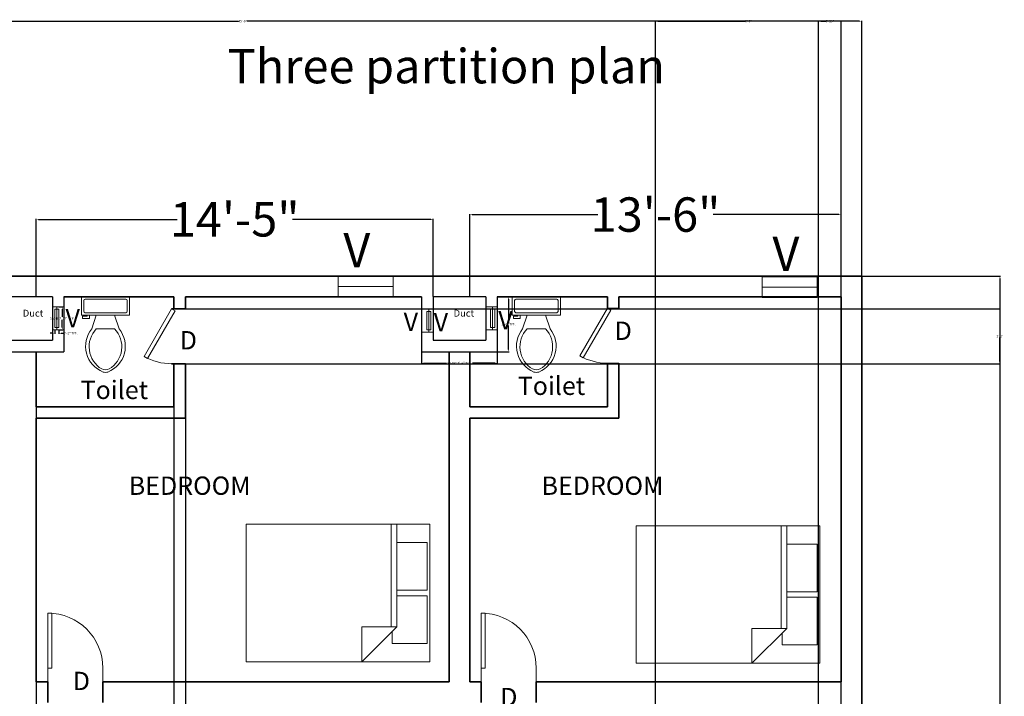
# Model space of a CAD drawing. Units: inches. Extents: x 371 to 1095, y -45 to 1219.
# Tile 18 of 18: x 666 to 1095, y 799 to 1094. Entities that reach past the tile are written whole.
import ezdxf

# ---------------------------------------------------------------- set-up
doc = ezdxf.new("R2010")
doc.units = ezdxf.units.IN
doc.header["$MEASUREMENT"] = 0
for name, color, linetype, lineweight in [('A-ANNO-DIMS', 2, 'Continuous', 18), ('A-ANNO-TEXT', 7, 'Continuous', 18), ('A-AREA-IDEN', 7, 'Continuous', 18), ('A-DOOR', 3, 'Continuous', 18), ('A-FLOR-FIXT', 9, 'Continuous', 18), ('A-FLOR-SHFT', 7, 'Continuous', 25), ('A-FURN', 254, 'Continuous', 18), ('A-GLAZ', 4, 'Continuous', 18), ('A-WALL', 40, 'Continuous', 35)]:
    doc.layers.add(name, color=color, linetype=linetype, lineweight=lineweight)
doc.styles.get("Standard").update_dxf_attribs({"font": 'arial.ttf'})
doc.dimstyles.get("Standard").update_dxf_attribs({"dimtxt": 1, "dimasz": 1, "dimexe": 0.18, "dimexo": 0.0625, "dimgap": 0.09, "dimtad": 0, "dimtih": 1, "dimtoh": 1, "dimdec": 0, "dimzin": 0, "dimdsep": 46, "dimlunit": 3, "dimtxsty": 'Standard', "dimcen": 0.09, "dimadec": 0, "dimazin": 0, "dimtfac": 1, "dimtdec": 0, "dimtofl": 0, "dimtmove": 0, "dimatfit": 3, "dimfxl": 1, "dimtolj": 1, "dimtzin": 0, "dimarcsym": 0})

# ---------------------------------------------------------------- blocks, each defined once
blk = doc.blocks.new('*U2')
for p, q in [((9.5, -6), (9.5, -2)), ((-10, -8.5), (-8, -8.5)), ((-10, -9.5), (-10, -8.5)), ((-8, -8.5), (-8, -8)), ((-7, -8), (-7, -9.5)), ((-4, -8), (-6, -14)), ((4, -8), (6, -14)), ((-7, -9.5), (-10, -9.5)), ((4, -14), (-4, -14))]:
    blk.add_line(p, q)
blk.add_lwpolyline([(10.5, -8), (10.5, 0), (-10.5, 0), (-10.5, -8)], close=True)
for points in [[(-9.5, -2), (-9.5, -6)], [(8.5, -1), (-8.5, -1)], [(-8.5, -7), (8.5, -7)]]:
    blk.add_lwpolyline(points)
for centre, radius, start, end in [((-8.62, -1.88), 0.884, 81.8699, 188.1301), ((8.62, -1.88), 0.884, 351.8699, 98.1301), ((-8.62, -6.12), 0.884, 171.8699, 278.1301), ((8.62, -6.12), 0.884, 261.8699, 8.1301), ((3.52, -21.58), 12.17, 141.4691, 247.9714), ((4.2, -21.82), 11.33, 136.3677, 238.9468), ((-3.52, -21.58), 12.17, 292.0284, 38.5307), ((-4.2, -21.82), 11.33, 301.053, 43.6321), ((0, -27.88), 4, 245.7318, 294.2682), ((0, -29), 4, 254.8605, 285.1395)]:
    blk.add_arc(centre, radius, start, end)
blk = doc.blocks.new('*U6')
for p, q in [((0, 0), (0, 6)), ((24, 0), (24, 6))]:
    blk.add_line(p, q)
blk.add_lwpolyline([(0, 0), (20.78, -12), (21.66, -10.48), (0.87, 1.52)], close=True)
blk.add_arc((0, 0), 24, 330, 0)
blk = doc.blocks.new('*U7')
for p, q in [((0, 0), (0, 5)), ((24, 0), (24, 5))]:
    blk.add_line(p, q)
blk.add_lwpolyline([(0, 0), (20.78, -12), (21.66, -10.48), (0.87, 1.52)], close=True)
blk.add_arc((0, 0), 24, 330, 0)
blk = doc.blocks.new('*U4')
for p, q in [((-24, 0), (-24, -6)), ((0, 0), (0, -6))]:
    blk.add_line(p, q)
blk.add_lwpolyline([(0, 0), (0, 24), (-1.75, 24), (-1.75, 0)], close=True)
blk.add_arc((0, 0), 24, 90, 180)
blk = doc.blocks.new('*D9')
at = {"layer": 'A-ANNO-DIMS', "color": 0, "lineweight": -2, "transparency": 16777216}
for p, q in [((672.81, 973.09), (672.81, 1006.96)), ((673.81, 1006.78), (734.16, 1006.78)), ((844.81, 1006.78), (784.46, 1006.78)), ((845.81, 973.09), (845.81, 1006.96))]:
    blk.add_line(p, q, dxfattribs=at)
at = {"layer": 'A-ANNO-DIMS', "color": 0, "transparency": 16777216}
for points in [[(673.81, 1006.95), (673.81, 1006.61), (672.81, 1006.78)], [(844.81, 1006.95), (844.81, 1006.61), (845.81, 1006.78)]]:
    blk.add_solid(points, dxfattribs=at)
at = {"layer": 'Defpoints', "color": 0, "transparency": 16777216}
for p in [(845.81, 1006.78), (672.81, 973.03), (845.81, 973.03)]:
    blk.add_point(p, dxfattribs=at)
at = {"layer": 'A-ANNO-DIMS', "color": 0, "transparency": 16777216, "insert": (759.31, 1006.78), "char_height": 1, "attachment_point": 5}
blk.add_mtext('\\A1;{\\H15x;14\'-5"}', dxfattribs=at)
blk = doc.blocks.new('*D10')
at = {"layer": 'A-ANNO-DIMS', "color": 0, "lineweight": -2, "transparency": 16777216}
for p, q in [((861.81, 973.2), (861.81, 1009.05)), ((1023.81, 973.09), (1023.81, 1009.05)), ((862.81, 1008.87), (917.66, 1008.87)), ((1022.81, 1008.87), (967.96, 1008.87))]:
    blk.add_line(p, q, dxfattribs=at)
at = {"layer": 'A-ANNO-DIMS', "color": 0, "transparency": 16777216}
for points in [[(862.81, 1009.03), (862.81, 1008.7), (861.81, 1008.87)], [(1022.81, 1009.03), (1022.81, 1008.7), (1023.81, 1008.87)]]:
    blk.add_solid(points, dxfattribs=at)
at = {"layer": 'Defpoints', "color": 0, "transparency": 16777216}
for p in [(1023.81, 1008.87), (861.81, 973.14), (1023.81, 973.03)]:
    blk.add_point(p, dxfattribs=at)
at = {"layer": 'A-ANNO-DIMS', "color": 0, "transparency": 16777216, "insert": (942.81, 1008.87), "char_height": 1, "attachment_point": 5}
blk.add_mtext('\\A1;{\\H15x;13\'-6"}', dxfattribs=at)
blk = doc.blocks.new('Bed - Queen')
for p, q in [((0, -80.00003), (0, 0)), ((0, 0), (59.99999, 0)), ((59.99999, 0), (59.99999, -80.00003)), ((7.99999, -1.2), (28.79998, -1.2)), ((7.99999, -14.4), (7.99999, -1.2)), ((28.79998, -1.2), (28.79998, -14.4)), ((31.19999, -1.2), (51.99999, -1.2)), ((31.19999, -14.4), (31.19999, -1.2)), ((51.99999, -1.2), (51.99999, -16.4)), ((0, -14.4), (44.8, -14.4)), ((44.8, -16.8), (0, -16.8)), ((59.99999, -29.6), (44.8, -14.4)), ((44.8, -14.4), (44.8, -29.6)), ((51.99999, -16.4), (46.79936, -16.4)), ((44.8, -29.6), (59.99999, -29.6)), ((59.99999, -80.00003), (0, -80.00003))]:
    blk.add_line(p, q)
blk = doc.blocks.new('VENT-24-REAR')
blk.add_line((0, 4.5), (24, 4.5))
blk.add_lwpolyline([(0, 9), (24, 9), (24, 0), (0, 0)], close=True)
blk = doc.blocks.new('VENT-DUCT-SASH')
blk.add_line((0.9, 10), (0.9, 0))
blk.add_lwpolyline([(1.79, 9), (1.79, 1), (0, 1), (0, 9)], close=True)
blk = doc.blocks.new('SHAFT-REAR')
for p, q in [((0, 24), (0, 0)), ((5, 24), (5, 5)), ((28, 24), (5, 24)), ((28, 24), (28, 5)), ((33, 24), (33, 0)), ((5, 5), (28, 5)), ((0, 0), (33, 0))]:
    blk.add_line(p, q)
blk = doc.blocks.new('*D42')
at = {"layer": 'A-ANNO-DIMS', "color": 0, "lineweight": -2, "transparency": 16777216}
for p, q in [((682.69, 968.59), (684.31, 968.59)), ((684.13, 967.59), (684.13, 964.19)), ((684.13, 959.59), (684.13, 962.98)), ((682.69, 958.59), (684.31, 958.59))]:
    blk.add_line(p, q, dxfattribs=at)
at = {"layer": 'A-ANNO-DIMS', "color": 0, "transparency": 16777216}
for points in [[(683.96, 967.59), (684.3, 967.59), (684.13, 968.59)], [(683.96, 959.59), (684.3, 959.59), (684.13, 958.59)]]:
    blk.add_solid(points, dxfattribs=at)
at = {"layer": 'Defpoints', "color": 0, "transparency": 16777216}
for p in [(682.63, 968.59), (684.13, 968.59), (682.63, 958.59)]:
    blk.add_point(p, dxfattribs=at)
at = {"layer": 'A-ANNO-DIMS', "color": 0, "transparency": 16777216, "insert": (684.13, 963.59), "char_height": 1, "attachment_point": 5}
blk.add_mtext('\\A1;SASH 0\'-10" TYP.', dxfattribs=at)
blk = doc.blocks.new('*D43')
at = {"layer": 'A-ANNO-DIMS', "color": 0, "lineweight": -2, "transparency": 16777216}
for p, q in [((680.84, 958.52), (680.84, 956.91)), ((682.63, 958.52), (682.63, 956.91)), ((679.84, 957.09), (678.84, 957.09)), ((683.63, 957.09), (684.63, 957.09))]:
    blk.add_line(p, q, dxfattribs=at)
at = {"layer": 'A-ANNO-DIMS', "color": 0, "transparency": 16777216}
for points in [[(679.84, 957.25), (679.84, 956.92), (680.84, 957.09)], [(683.63, 957.25), (683.63, 956.92), (682.63, 957.09)]]:
    blk.add_solid(points, dxfattribs=at)
at = {"layer": 'Defpoints', "color": 0, "transparency": 16777216}
for p in [(680.84, 958.59), (682.63, 958.59), (682.63, 957.09)]:
    blk.add_point(p, dxfattribs=at)
at = {"layer": 'A-ANNO-DIMS', "color": 0, "transparency": 16777216, "insert": (687.77, 957.09), "char_height": 1, "attachment_point": 5}
blk.add_mtext('\\A1;0\'-2" TYP.', dxfattribs=at)
blk = doc.blocks.new('*D46')
at = {"layer": 'A-ANNO-DIMS', "color": 0, "lineweight": -2, "transparency": 16777216}
for p, q in [((840.81, 948.96), (840.81, 943.9)), ((873.81, 948.96), (873.81, 943.9)), ((841.81, 944.08), (851.69, 944.08)), ((872.81, 944.08), (862.93, 944.08))]:
    blk.add_line(p, q, dxfattribs=at)
at = {"layer": 'A-ANNO-DIMS', "color": 0, "transparency": 16777216}
for points in [[(841.81, 944.24), (841.81, 943.91), (840.81, 944.08)], [(872.81, 944.24), (872.81, 943.91), (873.81, 944.08)]]:
    blk.add_solid(points, dxfattribs=at)
at = {"layer": 'Defpoints', "color": 0, "transparency": 16777216}
for p in [(840.81, 949.03), (873.81, 949.03), (873.81, 944.08)]:
    blk.add_point(p, dxfattribs=at)
at = {"layer": 'A-ANNO-DIMS', "color": 0, "transparency": 16777216, "insert": (857.31, 944.08), "char_height": 1, "attachment_point": 5}
blk.add_mtext('\\A1;SHAFT 2\'-9" TYP.', dxfattribs=at)
blk = doc.blocks.new('*D47')
at = {"layer": 'A-ANNO-DIMS', "color": 0, "lineweight": -2, "transparency": 16777216}
for p, q in [((873.87, 973.03), (878.94, 973.03)), ((878.76, 972.03), (878.76, 961.63)), ((878.76, 950.03), (878.76, 960.42)), ((873.87, 949.03), (878.94, 949.03))]:
    blk.add_line(p, q, dxfattribs=at)
at = {"layer": 'A-ANNO-DIMS', "color": 0, "transparency": 16777216}
for points in [[(878.59, 972.03), (878.92, 972.03), (878.76, 973.03)], [(878.59, 950.03), (878.92, 950.03), (878.76, 949.03)]]:
    blk.add_solid(points, dxfattribs=at)
at = {"layer": 'Defpoints', "color": 0, "transparency": 16777216}
for p in [(873.81, 973.03), (878.76, 973.03), (873.81, 949.03)]:
    blk.add_point(p, dxfattribs=at)
at = {"layer": 'A-ANNO-DIMS', "color": 0, "transparency": 16777216, "insert": (878.76, 961.03), "char_height": 1, "attachment_point": 5}
blk.add_mtext('\\A1;2\'-0" TYP.', dxfattribs=at)
blk = doc.blocks.new('*D50')
at = {"layer": 'A-ANNO-DIMS', "color": 0, "lineweight": -2, "transparency": 16777216}
for p, q in [((492.81, 982.09), (492.81, 1093.41)), ((493.81, 1093.23), (760.98, 1093.23)), ((1031.81, 1093.23), (764.64, 1093.23)), ((1032.81, 982.09), (1032.81, 1093.41))]:
    blk.add_line(p, q, dxfattribs=at)
at = {"layer": 'A-ANNO-DIMS', "color": 0, "transparency": 16777216}
for points in [[(493.81, 1093.39), (493.81, 1093.06), (492.81, 1093.23)], [(1031.81, 1093.39), (1031.81, 1093.06), (1032.81, 1093.23)]]:
    blk.add_solid(points, dxfattribs=at)
at = {"layer": 'Defpoints', "color": 0, "transparency": 16777216}
for p in [(1032.81, 1093.23), (492.81, 982.03), (1032.81, 982.03)]:
    blk.add_point(p, dxfattribs=at)
at = {"layer": 'A-ANNO-DIMS', "color": 0, "transparency": 16777216, "insert": (762.81, 1093.23), "char_height": 1, "attachment_point": 5}
blk.add_mtext('\\A1;45\'-0"', dxfattribs=at)
blk = doc.blocks.new('*D51')
at = {"layer": 'A-ANNO-DIMS', "color": 0, "lineweight": -2, "transparency": 16777216}
for p, q in [((1032.87, 982.03), (1093.19, 982.03)), ((1093.01, 981.03), (1093.01, 532.63)), ((1093.01, 83.03), (1093.01, 531.42)), ((1032.87, 82.03), (1093.19, 82.03))]:
    blk.add_line(p, q, dxfattribs=at)
at = {"layer": 'A-ANNO-DIMS', "color": 0, "transparency": 16777216}
for points in [[(1092.84, 981.03), (1093.17, 981.03), (1093.01, 982.03)], [(1092.84, 83.03), (1093.17, 83.03), (1093.01, 82.03)]]:
    blk.add_solid(points, dxfattribs=at)
at = {"layer": 'Defpoints', "color": 0, "transparency": 16777216}
for p in [(1032.81, 982.03), (1093.01, 982.03), (1032.81, 82.03)]:
    blk.add_point(p, dxfattribs=at)
at = {"layer": 'A-ANNO-DIMS', "color": 0, "transparency": 16777216, "insert": (1093.01, 532.03), "char_height": 1, "attachment_point": 5}
blk.add_mtext('\\A1;75\'-0"', dxfattribs=at)
blk = doc.blocks.new('*D54')
at = {"layer": 'A-ANNO-DIMS', "color": 0, "lineweight": -2, "transparency": 16777216}
for p, q in [((672.81, 924.96), (672.81, -43.83)), ((732.81, 924.96), (732.81, -43.83)), ((673.81, -43.65), (701.39, -43.65)), ((731.81, -43.65), (704.23, -43.65))]:
    blk.add_line(p, q, dxfattribs=at)
at = {"layer": 'A-ANNO-DIMS', "color": 0, "transparency": 16777216}
for points in [[(673.81, -43.48), (673.81, -43.82), (672.81, -43.65)], [(731.81, -43.48), (731.81, -43.82), (732.81, -43.65)]]:
    blk.add_solid(points, dxfattribs=at)
at = {"layer": 'Defpoints', "color": 0, "transparency": 16777216}
for p in [(672.81, 925.03), (732.81, 925.03), (732.81, -43.65)]:
    blk.add_point(p, dxfattribs=at)
at = {"layer": 'A-ANNO-DIMS', "color": 0, "transparency": 16777216, "insert": (702.81, -43.65), "char_height": 1, "attachment_point": 5}
blk.add_mtext('\\A1;5\'-0"', dxfattribs=at)
blk = doc.blocks.new('*D56')
at = {"layer": 'A-ANNO-DIMS', "color": 0, "lineweight": -2, "transparency": 16777216}
for p, q in [((737.87, 967.8), (1093.19, 967.8)), ((1093.01, 966.8), (1093.01, 956.4)), ((1093.01, 944.8), (1093.01, 955.2)), ((737.87, 943.8), (1093.19, 943.8))]:
    blk.add_line(p, q, dxfattribs=at)
at = {"layer": 'A-ANNO-DIMS', "color": 0, "transparency": 16777216}
for points in [[(1092.84, 966.8), (1093.17, 966.8), (1093.01, 967.8)], [(1092.84, 944.8), (1093.17, 944.8), (1093.01, 943.8)]]:
    blk.add_solid(points, dxfattribs=at)
at = {"layer": 'Defpoints', "color": 0, "transparency": 16777216}
for p in [(737.81, 967.8), (1093.01, 967.8), (737.81, 943.8)]:
    blk.add_point(p, dxfattribs=at)
at = {"layer": 'A-ANNO-DIMS', "color": 0, "transparency": 16777216, "insert": (1093.01, 955.8), "char_height": 1, "attachment_point": 5}
blk.add_mtext('\\A1;2\'-0"', dxfattribs=at)
blk = doc.blocks.new('*D57')
at = {"layer": 'A-ANNO-DIMS', "color": 0, "lineweight": -2, "transparency": 16777216}
for p, q in [((732.81, 924.96), (732.81, -43.83)), ((737.81, 919.96), (737.81, -43.83)), ((731.81, -43.65), (730.81, -43.65)), ((738.81, -43.65), (739.81, -43.65))]:
    blk.add_line(p, q, dxfattribs=at)
at = {"layer": 'A-ANNO-DIMS', "color": 0, "transparency": 16777216}
for points in [[(731.81, -43.48), (731.81, -43.82), (732.81, -43.65)], [(738.81, -43.48), (738.81, -43.82), (737.81, -43.65)]]:
    blk.add_solid(points, dxfattribs=at)
at = {"layer": 'Defpoints', "color": 0, "transparency": 16777216}
for p in [(732.81, 925.03), (737.81, 920.03), (732.81, -43.65)]:
    blk.add_point(p, dxfattribs=at)
at = {"layer": 'A-ANNO-DIMS', "color": 0, "transparency": 16777216, "insert": (735.31, -43.65), "char_height": 1, "attachment_point": 5}
blk.add_mtext('\\A1;0\'-5"', dxfattribs=at)
blk = doc.blocks.new('*D63')
at = {"layer": 'A-ANNO-DIMS', "color": 0, "lineweight": -2, "transparency": 16777216}
for p, q in [((942.81, 580.09), (942.81, 1093.41)), ((943.81, 1093.23), (981.89, 1093.23)), ((1022.81, 1093.23), (984.73, 1093.23)), ((1023.81, 580.09), (1023.81, 1093.41))]:
    blk.add_line(p, q, dxfattribs=at)
at = {"layer": 'A-ANNO-DIMS', "color": 0, "transparency": 16777216}
for points in [[(943.81, 1093.39), (943.81, 1093.06), (942.81, 1093.23)], [(1022.81, 1093.39), (1022.81, 1093.06), (1023.81, 1093.23)]]:
    blk.add_solid(points, dxfattribs=at)
at = {"layer": 'Defpoints', "color": 0, "transparency": 16777216}
for p in [(1023.81, 1093.23), (942.81, 580.03), (1023.81, 580.03)]:
    blk.add_point(p, dxfattribs=at)
at = {"layer": 'A-ANNO-DIMS', "color": 0, "transparency": 16777216, "insert": (983.31, 1093.23), "char_height": 1, "attachment_point": 5}
blk.add_mtext('\\A1;6\'-9"', dxfattribs=at)
blk = doc.blocks.new('*D64')
at = {"layer": 'A-ANNO-DIMS', "color": 0, "lineweight": -2, "transparency": 16777216}
for p, q in [((1013.84, 464.01), (1013.84, 1093.41)), ((1014.84, 1093.23), (1017.01, 1093.23)), ((1022.81, 1093.23), (1020.63, 1093.23)), ((1023.81, 451.09), (1023.81, 1093.41))]:
    blk.add_line(p, q, dxfattribs=at)
at = {"layer": 'A-ANNO-DIMS', "color": 0, "transparency": 16777216}
for points in [[(1014.84, 1093.39), (1014.84, 1093.06), (1013.84, 1093.23)], [(1022.81, 1093.39), (1022.81, 1093.06), (1023.81, 1093.23)]]:
    blk.add_solid(points, dxfattribs=at)
at = {"layer": 'Defpoints', "color": 0, "transparency": 16777216}
for p in [(1023.81, 1093.23), (1013.84, 463.94), (1023.81, 451.03)]:
    blk.add_point(p, dxfattribs=at)
at = {"layer": 'A-ANNO-DIMS', "color": 0, "transparency": 16777216, "insert": (1018.82, 1093.23), "char_height": 1, "attachment_point": 5}
blk.add_mtext('\\A1;0\'-10"', dxfattribs=at)

msp = doc.modelspace()

# ---------------------------------------------------------------- linework, layer by layer
at = {"layer": 'A-FLOR-SHFT'}
msp.add_line((868.81, 973.03), (845.81, 973.03), dxfattribs=at)
at = {"layer": 'A-GLAZ'}
for points in [[(684.81, 968.59), (684.81, 958.59), (679.81, 958.59), (679.81, 968.59)], [(845.81, 967.58), (845.81, 957.58), (840.81, 957.58), (840.81, 967.58)], [(873.81, 968.61), (873.81, 958.61), (868.81, 958.61), (868.81, 968.61)]]:
    msp.add_lwpolyline(points, close=True, dxfattribs=at)
at = {"layer": 'A-WALL'}
for p, q in [((1032.81, 982.03), (492.81, 982.03)), ((1032.81, 82.03), (1032.81, 982.03)), ((684.81, 973.03), (732.81, 973.03)), ((732.81, 973.03), (684.81, 973.03)), ((732.81, 973.03), (732.81, 967.8)), ((737.81, 973.03), (737.81, 967.8)), ((737.81, 973.03), (840.81, 973.03)), ((840.81, 973.03), (737.81, 973.03)), ((921.81, 973.03), (873.81, 973.03)), ((873.81, 973.03), (921.81, 973.03)), ((921.81, 968.03), (921.81, 973.03)), ((921.81, 968.03), (921.81, 973.03)), ((1023.81, 973.03), (926.81, 973.03)), ((926.81, 973.03), (1023.81, 973.03)), ((926.81, 968.03), (926.81, 973.03)), ((1023.81, 805.03), (1023.81, 973.03)), ((731.81, 967.8), (737.81, 967.8)), ((672.81, 949.02), (672.81, 925.03)), ((852.81, 805.03), (852.81, 949.02)), ((861.81, 925.03), (861.81, 949.02)), ((737.81, 943.8), (731.81, 943.8)), ((732.81, 943.8), (732.81, 925.03)), ((737.81, 943.8), (737.81, 920.03)), ((921.81, 925.03), (921.81, 944.03)), ((926.81, 920.03), (926.81, 944.03)), ((672.81, 925.03), (732.81, 925.03)), ((861.81, 925.03), (921.81, 925.03)), ((861.81, 925.03), (921.81, 925.03)), ((672.81, 920.03), (737.81, 920.03)), ((672.81, 920.03), (672.81, 805.03)), ((861.81, 920.03), (926.81, 920.03)), ((861.81, 805.03), (861.81, 920.03)), ((672.81, 805.03), (677.81, 805.03)), ((677.81, 796.03), (677.81, 805.03)), ((701.81, 805.03), (701.81, 796.03)), ((701.81, 805.03), (852.81, 805.03)), ((861.81, 805.03), (866.81, 805.03)), ((866.81, 805.03), (866.81, 796.03)), ((890.81, 805.03), (890.81, 796.03)), ((890.81, 805.03), (1023.81, 805.03))]:
    msp.add_line(p, q, dxfattribs=at)

# ---------------------------------------------------------------- block references
at = {"layer": 'A-DOOR', "rotation": 270}
for name, p in [('*U6', (731.81, 967.8)), ('*U7', (921.81, 968.03))]:
    msp.add_blockref(name, p, dxfattribs=at)
at = {"layer": 'A-DOOR', "xscale": -1}
for p in [(677.81, 811.03), (866.81, 811.03)]:
    msp.add_blockref('*U4', p, dxfattribs=at)
at = {"layer": 'A-FLOR-FIXT'}
for p in [(702.96, 973.03), (890.83, 973.03)]:
    msp.add_blockref('*U2', p, dxfattribs=at)
at = {"layer": 'A-FLOR-SHFT'}
for p in [(651.81, 949.02), (840.81, 949.02)]:
    msp.add_blockref('SHAFT-REAR', p, dxfattribs=at)
at = {"layer": 'A-FURN', "rotation": 270}
for p in [(844.37, 873.79), (1014.42, 873.11)]:
    msp.add_blockref('Bed - Queen', p, dxfattribs=at)
at = {"layer": 'A-GLAZ'}
for name, p in [('VENT-24-REAR', (804.36, 972.98)), ('VENT-24-REAR', (989.32, 972.72)), ('VENT-DUCT-SASH', (680.84, 958.59)), ('VENT-DUCT-SASH', (843.03, 957.58)), ('VENT-DUCT-SASH', (870.88, 958.61))]:
    msp.add_blockref(name, p, dxfattribs=at)

# ---------------------------------------------------------------- texts
at = {"layer": 'A-ANNO-TEXT', "attachment_point": 1}
for s, width, insert, char_height in [('Three partition plan', 211.3773, (756.26, 1081.12), 15), ('V', 17.4938, (806.68, 1000.88), 15), ('V', 17.4938, (993.77, 999.26), 15), ('V', 17.4938, (685.54, 967.64), 8), ('V', 17.4938, (832.98, 966.09), 8), ('V', 17.4938, (874.26, 966.77), 8), ('V', 17.4938, (846.08, 965.96), 8), ('D', 17.4938, (924.98, 962.17), 8), ('D', 17.4938, (735.34, 958.04), 8), ('D', 17.4938, (688.7, 809.41), 8), ('D', 17.4938, (875.09, 802.38), 8)]:
    msp.add_mtext_dynamic_manual_height_columns(s, width=width, gutter_width=1, heights=[0], dxfattribs=dict(at, insert=insert, char_height=char_height))
at = {"layer": 'A-AREA-IDEN', "attachment_point": 1}
for s, width, insert, char_height in [('Duct', 31.9108, (666.9, 967.35), 3), ('Duct', 31.9108, (854.76, 967.35), 3), ('Toilet', 31.9108, (692.14, 936.39), 8), ('Toilet', 31.9108, (882.75, 938.18), 8), ('BEDROOM', 53.6318, (713.13, 894.6), 8), ('BEDROOM', 53.6318, (893.13, 894.6), 8)]:
    msp.add_mtext_dynamic_manual_height_columns(s, width=width, gutter_width=1, heights=[0], dxfattribs=dict(at, insert=insert, char_height=char_height))

# ---------------------------------------------------------------- dimensions: what is measured, and where the dimension line sits
at = {"layer": 'A-ANNO-DIMS'}
for base, p1, p2, picture, middle in [((1032.81, 1093.23), (492.81, 982.03), (1032.81, 982.03), '*D50', (762.81, 1093.23)), ((1023.81, 1093.23), (942.81, 580.03), (1023.81, 580.03), '*D63', (983.31, 1093.23)), ((1023.81, 1093.23), (1013.84, 463.94), (1023.81, 451.03), '*D64', (1018.82, 1093.23)), ((732.81, -43.65), (672.81, 925.03), (732.81, 925.03), '*D54', (702.81, -43.65)), ((732.81, -43.65), (737.81, 920.03), (732.81, 925.03), '*D57', (735.31, -43.65))]:
    dim = msp.add_linear_dim(base=base, p1=p1, p2=p2, dimstyle='Standard', override={"dimdec": 1, "dimlfac": 1, "dimrnd": 0, "dimzin": 1, "dimdsep": 46, "dimlunit": 4, "dimfrac": 2}, dxfattribs=at)
    dim.commit()
    dim.dimension.update_dxf_attribs({"geometry": picture, "text_midpoint": middle})
for base, p1, p2, text, override, picture, middle in [((845.81, 1006.78), (672.81, 973.03), (845.81, 973.03), '{\\H15x;<>}', {"dimclrd": 0, "dimclre": 0, "dimclrt": 0}, '*D9', (759.31, 1006.78)), ((1023.81, 1008.87), (861.81, 973.14), (1023.81, 973.03), '{\\H15x;<>}', {"dimclrd": 0, "dimclre": 0, "dimclrt": 0}, '*D10', (942.81, 1008.87)), ((682.63, 957.09), (680.84, 958.59), (682.63, 958.59), '<> TYP.', {"dimdec": 1, "dimlfac": 1, "dimrnd": 0, "dimzin": 1, "dimdsep": 46, "dimlunit": 4, "dimfrac": 2}, '*D43', (687.77, 957.09)), ((873.81, 944.08), (840.81, 949.02), (873.81, 949.02), 'SHAFT <> TYP.', {"dimdec": 1, "dimlfac": 1, "dimrnd": 0, "dimzin": 1, "dimdsep": 46, "dimlunit": 4, "dimfrac": 2}, '*D46', (857.31, 944.08))]:
    dim = msp.add_linear_dim(base=base, p1=p1, p2=p2, text=text, dimstyle='Standard', override=override, dxfattribs=at)
    dim.commit()
    dim.dimension.update_dxf_attribs({"geometry": picture, "text_midpoint": middle})
for base, p1, p2, picture, middle in [((1093.01, 982.03), (1032.81, 82.03), (1032.81, 982.03), '*D51', (1093.01, 532.03)), ((1093.01, 967.8), (737.81, 943.8), (737.81, 967.8), '*D56', (1093.01, 955.8))]:
    dim = msp.add_linear_dim(base=base, p1=p1, p2=p2, angle=90, dimstyle='Standard', override={"dimdec": 1, "dimlfac": 1, "dimrnd": 0, "dimzin": 1, "dimdsep": 46, "dimlunit": 4, "dimfrac": 2}, dxfattribs=at)
    dim.commit()
    dim.dimension.update_dxf_attribs({"geometry": picture, "text_midpoint": middle})
for base, p1, p2, text, picture, middle in [((878.76, 973.03), (873.81, 949.02), (873.81, 973.03), '<> TYP.', '*D47', (878.76, 961.03)), ((684.13, 968.59), (682.63, 958.59), (682.63, 968.59), 'SASH <> TYP.', '*D42', (684.13, 963.59))]:
    dim = msp.add_linear_dim(base=base, p1=p1, p2=p2, angle=90, text=text, dimstyle='Standard', override={"dimdec": 1, "dimlfac": 1, "dimrnd": 0, "dimzin": 1, "dimdsep": 46, "dimlunit": 4, "dimfrac": 2}, dxfattribs=at)
    dim.commit()
    dim.dimension.update_dxf_attribs({"geometry": picture, "text_midpoint": middle})

doc.saveas('drawing.dxf')
